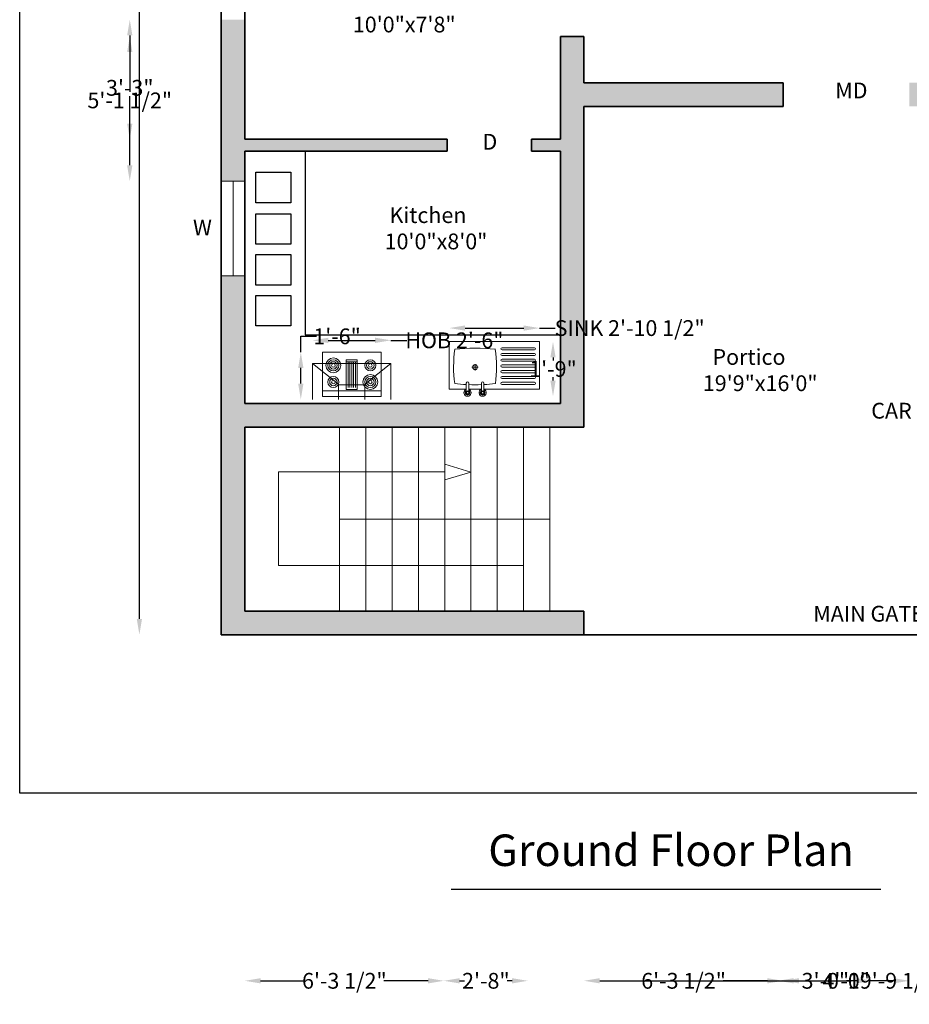
# Model space of a CAD drawing. Units: inches. Extents: x 1054 to 1577, y 4847 to 5610.
# Tile 1 of 5: x 1054 to 1393, y 4847 to 5221. Entities that reach past the tile are written whole.
import ezdxf

# ---------------------------------------------------------------- set-up
doc = ezdxf.new("R2010")
doc.units = ezdxf.units.IN
doc.header["$MEASUREMENT"] = 0
for name, color, linetype, lineweight in [('A-ANNO-DIMS', 2, 'Continuous', 18), ('A-ANNO-TEXT', 7, 'Continuous', 18), ('A-ANNO-TTLB', 7, 'Continuous', 25), ('A-AREA-IDEN', 7, 'Continuous', 18), ('A-EQPM', 8, 'Continuous', 18), ('A-FLOR-CASE', 7, 'Continuous', 25), ('A-FLOR-FIXT', 8, 'Continuous', 18), ('A-FLOR-STRS', 7, 'Continuous', 18), ('A-GLAZ', 4, 'Continuous', 18), ('A-WALL', 7, 'Continuous', 35)]:
    doc.layers.add(name, color=color, linetype=linetype, lineweight=lineweight)
doc.layers.add('A-WALL-PATT', color=240, linetype='Continuous', lineweight=13, true_color=0xed1f24)
doc.styles.get("Standard").update_dxf_attribs({"font": 'arial.ttf'})
doc.dimstyles.get("Standard").update_dxf_attribs({"dimtxt": 6, "dimasz": 6, "dimexe": 0.18, "dimexo": 0.0625, "dimgap": 0.09, "dimtad": 0, "dimtih": 1, "dimtoh": 1, "dimdec": 1, "dimzin": 0, "dimdsep": 46, "dimlunit": 3, "dimtxsty": 'Standard', "dimcen": 0.09, "dimse1": 1, "dimse2": 1, "dimadec": 0, "dimazin": 0, "dimtfac": 1, "dimtdec": 1, "dimtofl": 0, "dimtmove": 0, "dimatfit": 3, "dimfxl": 1, "dimtolj": 1, "dimtzin": 0, "dimarcsym": 0})

# ---------------------------------------------------------------- blocks, each defined once
blk = doc.blocks.new('chimmne')
for p, q in [((17.89, 6.07), (-18.11, 6.07)), ((-18.11, 6.07), (-18.11, -10.43)), ((-6.16, -3.43), (-18.11, 6.07)), ((5.94, -3.43), (17.89, 6.07)), ((17.89, 6.07), (17.89, -10.43)), ((-6.16, -3.43), (-6.16, -10.43)), ((5.94, -3.82), (-6.16, -3.82)), ((5.94, -3.43), (5.94, -10.43))]:
    blk.add_line(p, q)
for points in [[(-13.61, -9.12), (-13.61, 11.28), (13.39, 11.28), (13.39, -9.12)], [(-2.66, -5.87), (-2.66, 7.73), (2.44, 7.73), (2.44, -5.87)]]:
    blk.add_lwpolyline(points, close=True)
for points in [[(-2.66, 6.88), (2.44, 6.88)], [(-1.81, 6.88), (-1.81, -5.02)], [(-0.96, -5.02), (-0.96, 6.88)], [(-0.11, 6.88), (-0.11, -5.02)], [(0.74, -5.02), (0.74, 6.88)], [(1.59, 6.88), (1.59, -5.02)], [(13.39, -6.57), (-13.61, -6.57)]]:
    blk.add_lwpolyline(points)
for centre, radius in [((-8.55, 5.18), 3.4), ((-8.55, 5.18), 2.55), ((-8.55, 5.18), 1.7), ((-8.55, 5.18), 0.85), ((8.44, 5.18), 2.55), ((8.44, 5.18), 1.7), ((8.44, 5.18), 0.85), ((-8.55, -2.47), 2.55), ((8.44, -2.47), 3.4), ((8.44, -2.47), 2.55), ((-8.55, -2.47), 1.7), ((-8.55, -2.47), 0.85), ((8.44, -2.47), 1.7), ((8.44, -2.47), 0.85)]:
    blk.add_circle(centre, radius)
blk = doc.blocks.new('A$C799204C7')
for p, q in [((0, 34.2), (17.99, 34.2)), ((0, 0), (0, 34.2)), ((17.99, 13.08), (17.99, 34.2)), ((2.32, 20.01), (2.32, 32.27)), ((3.13, 20.01), (3.13, 32.27)), ((4.48, 20.01), (4.48, 32.27)), ((5.29, 20.01), (5.29, 32.27)), ((6.64, 20.01), (6.64, 32.27)), ((7.45, 20.01), (7.45, 32.27)), ((8.85, 20.01), (8.85, 32.27)), ((9.66, 20.01), (9.66, 32.27)), ((11.01, 20.01), (11.01, 32.27)), ((11.82, 20.01), (11.82, 32.27)), ((13.22, 20.01), (13.22, 32.27)), ((14.03, 20.01), (14.03, 32.27)), ((15.42, 20.01), (15.42, 32.27)), ((16.24, 20.01), (16.24, 32.27)), ((18.59, 13.08), (15.71, 13.08)), ((15.71, 12.17), (18.59, 12.17)), ((17.99, 7.36), (17.99, 12.17)), ((8.52, 9.77), (10.9, 9.77)), ((9.73, 11), (9.73, 8.54)), ((18.59, 7.36), (15.71, 7.36)), ((15.71, 6.45), (18.59, 6.45)), ((17.99, 0), (17.99, 6.45)), ((0, 0), (17.99, 0))]:
    blk.add_line(p, q)
for centre, radius in [((19.38, 12.62), 0.684), ((19.38, 12.62), 0.456), ((9.7, 9.77), 0.916), ((19.38, 6.91), 0.684), ((19.38, 6.91), 0.456)]:
    blk.add_circle(centre, radius)
for centre, radius, start, end in [((2.72, 32.27), 0.407, 0, 180), ((4.88, 32.27), 0.407, 0, 180), ((7.05, 32.27), 0.407, 0, 180), ((9.25, 32.27), 0.407, 0, 180), ((11.42, 32.27), 0.407, 0, 180), ((13.62, 32.27), 0.407, 0, 180), ((15.83, 32.27), 0.407, 0, 180), ((2.72, 20.01), 0.407, 180, 0), ((4.88, 20.01), 0.407, 180, 0), ((7.05, 20.01), 0.407, 180, 0), ((9.25, 20.01), 0.407, 180, 0), ((11.42, 20.01), 0.407, 180, 0), ((13.62, 20.01), 0.407, 180, 0), ((15.83, 20.01), 0.407, 180, 0), ((67.33, 9.77), 64.88, 173.1952, 186.8048), ((9.53, -30.19), 48.1, 82.3437, 97.8966), ((-48.51, 9.77), 64.88, 2.9208, 6.8048), ((15.71, 12.62), 0.456, 90, 270), ((-48.51, 9.77), 64.88, 357.8723, 2.115), ((19.38, 12.62), 1.37, 199.6514, 160.3603), ((19.38, 12.62), 0.911, 210.3431, 149.7554), ((19.38, 6.91), 1.37, 199.6514, 160.3603), ((19.38, 6.91), 0.911, 210.3431, 149.7554), ((15.71, 6.91), 0.456, 90, 270), ((-48.51, 9.77), 64.88, 353.1952, 357.0665), ((9.53, 49.73), 48.1, 262.1034, 277.6563)]:
    blk.add_arc(centre, radius, start, end)
blk = doc.blocks.new('*D5')
at = {"layer": 'A-ANNO-DIMS', "color": 0, "lineweight": -2, "transparency": 16777216}
for p, q in [((1099.63, 5521.48), (1099.63, 5260.62)), ((1099.63, 4993.48), (1099.63, 5254.34))]:
    blk.add_line(p, q, dxfattribs=at)
at = {"layer": 'A-ANNO-DIMS', "color": 0, "transparency": 16777216}
for points in [[(1098.63, 5521.48), (1100.63, 5521.48), (1099.63, 5527.48)], [(1098.63, 4993.48), (1100.63, 4993.48), (1099.63, 4987.48)]]:
    blk.add_solid(points, dxfattribs=at)
at = {"layer": 'Defpoints', "color": 0, "transparency": 16777216}
for p in [(1130.77, 5527.48), (1099.63, 4987.48), (1130.77, 4987.48)]:
    blk.add_point(p, dxfattribs=at)
at = {"layer": 'A-ANNO-DIMS', "color": 0, "transparency": 16777216, "insert": (1099.63, 5257.48), "char_height": 6, "attachment_point": 5}
blk.add_mtext("\\A1;45'", dxfattribs=at)
blk = doc.blocks.new('WINDOW-36IN')
for p, q in [((0, 9), (0, 0)), ((36, 9), (0, 9)), ((36, 0), (36, 9)), ((36, 4.5), (0, 4.5)), ((0, 0), (36, 0))]:
    blk.add_line(p, q)
blk = doc.blocks.new('*D18')
at = {"layer": 'A-ANNO-DIMS', "color": 0, "lineweight": -2, "transparency": 16777216}
for p, q in [((1171.51, 5099.49), (1189.32, 5099.49)), ((1195.32, 5099.49), (1201.32, 5099.49))]:
    blk.add_line(p, q, dxfattribs=at)
at = {"layer": 'A-ANNO-DIMS', "color": 0, "transparency": 16777216}
for points in [[(1171.51, 5100.49), (1171.51, 5098.49), (1165.51, 5099.49)], [(1189.32, 5100.49), (1189.32, 5098.49), (1195.32, 5099.49)]]:
    blk.add_solid(points, dxfattribs=at)
at = {"layer": 'Defpoints', "color": 0, "transparency": 16777216}
for p in [(1195.32, 5099.49), (1165.51, 5095.02), (1195.32, 5095.02)]:
    blk.add_point(p, dxfattribs=at)
at = {"layer": 'A-ANNO-DIMS', "color": 0, "transparency": 16777216, "insert": (1219.47, 5099.49), "char_height": 6, "attachment_point": 5}
blk.add_mtext('\\A1;HOB 2\'-6"', dxfattribs=at)
blk = doc.blocks.new('*D19')
at = {"layer": 'A-ANNO-DIMS', "color": 0, "lineweight": -2, "transparency": 16777216}
for p, q in [((1161.04, 5095.02), (1161.04, 5101.02)), ((1161.04, 5101.02), (1167.04, 5101.02)), ((1161.04, 5083.04), (1161.04, 5089.02))]:
    blk.add_line(p, q, dxfattribs=at)
at = {"layer": 'A-ANNO-DIMS', "color": 0, "transparency": 16777216}
for points in [[(1160.04, 5089.02), (1162.04, 5089.02), (1161.04, 5095.02)], [(1160.04, 5083.04), (1162.04, 5083.04), (1161.04, 5077.04)]]:
    blk.add_solid(points, dxfattribs=at)
at = {"layer": 'Defpoints', "color": 0, "transparency": 16777216}
for p in [(1161.04, 5095.02), (1165.51, 5095.02), (1165.51, 5077.04)]:
    blk.add_point(p, dxfattribs=at)
at = {"layer": 'A-ANNO-DIMS', "color": 0, "transparency": 16777216, "insert": (1174.83, 5101.02), "char_height": 6, "attachment_point": 5}
blk.add_mtext('\\A1;1\'-6"', dxfattribs=at)
blk = doc.blocks.new('*D20')
at = {"layer": 'A-ANNO-DIMS', "color": 0, "lineweight": -2, "transparency": 16777216}
for p, q in [((1223.53, 5104.16), (1245.84, 5104.16)), ((1251.84, 5104.16), (1257.84, 5104.16))]:
    blk.add_line(p, q, dxfattribs=at)
at = {"layer": 'A-ANNO-DIMS', "color": 0, "transparency": 16777216}
for points in [[(1223.53, 5105.16), (1223.53, 5103.16), (1217.53, 5104.16)], [(1245.84, 5105.16), (1245.84, 5103.16), (1251.84, 5104.16)]]:
    blk.add_solid(points, dxfattribs=at)
at = {"layer": 'Defpoints', "color": 0, "transparency": 16777216}
for p in [(1251.84, 5104.16), (1217.53, 5099.01), (1251.84, 5099.01)]:
    blk.add_point(p, dxfattribs=at)
at = {"layer": 'A-ANNO-DIMS', "color": 0, "transparency": 16777216, "insert": (1286.15, 5104.16), "char_height": 6, "attachment_point": 5}
blk.add_mtext('\\A1;SINK 2\'-10 1/2"', dxfattribs=at)
blk = doc.blocks.new('*D21')
at = {"layer": 'A-ANNO-DIMS', "color": 0, "lineweight": -2, "transparency": 16777216}
for p, q in [((1256.98, 5093.01), (1256.98, 5091.76)), ((1256.98, 5084.2), (1256.98, 5085.45))]:
    blk.add_line(p, q, dxfattribs=at)
at = {"layer": 'A-ANNO-DIMS', "color": 0, "transparency": 16777216}
for points in [[(1255.98, 5093.01), (1257.98, 5093.01), (1256.98, 5099.01)], [(1255.98, 5084.2), (1257.98, 5084.2), (1256.98, 5078.2)]]:
    blk.add_solid(points, dxfattribs=at)
at = {"layer": 'Defpoints', "color": 0, "transparency": 16777216}
for p in [(1251.84, 5099.01), (1251.84, 5078.2), (1256.98, 5078.2)]:
    blk.add_point(p, dxfattribs=at)
at = {"layer": 'A-ANNO-DIMS', "color": 0, "transparency": 16777216, "insert": (1256.98, 5088.6), "char_height": 6, "attachment_point": 5}
blk.add_mtext('\\A1;1\'-9"', dxfattribs=at)
blk = doc.blocks.new('*D22')
at = {"layer": 'A-ANNO-DIMS', "color": 0, "lineweight": -2, "transparency": 16777216}
for p, q in [((1397.97, 5125.61), (1397.97, 5075.91)), ((1397.97, 5019.83), (1397.97, 5069.53))]:
    blk.add_line(p, q, dxfattribs=at)
at = {"layer": 'A-ANNO-DIMS', "color": 0, "transparency": 16777216}
for points in [[(1396.97, 5125.61), (1398.97, 5125.61), (1397.97, 5131.61)], [(1396.97, 5019.83), (1398.97, 5019.83), (1397.97, 5013.83)]]:
    blk.add_solid(points, dxfattribs=at)
at = {"layer": 'Defpoints', "color": 0, "transparency": 16777216}
for p in [(1415.63, 5131.61), (1397.97, 5013.83), (1415.63, 5013.83)]:
    blk.add_point(p, dxfattribs=at)
at = {"layer": 'A-ANNO-DIMS', "color": 0, "transparency": 16777216, "insert": (1397.97, 5072.72), "char_height": 6, "attachment_point": 5}
blk.add_mtext('\\A1;CAR 9\'-10"', dxfattribs=at)
blk = doc.blocks.new('*D24')
at = {"layer": 'A-ANNO-DIMS', "color": 0, "lineweight": -2, "transparency": 16777216}
for p, q in [((1350.52, 4855.83), (1360.34, 4855.83)), ((1386.52, 4855.83), (1376.71, 4855.83))]:
    blk.add_line(p, q, dxfattribs=at)
at = {"layer": 'A-ANNO-DIMS', "color": 0, "transparency": 16777216}
for points in [[(1350.52, 4856.83), (1350.52, 4854.83), (1344.52, 4855.83)], [(1386.52, 4856.83), (1386.52, 4854.83), (1392.52, 4855.83)]]:
    blk.add_solid(points, dxfattribs=at)
at = {"layer": 'Defpoints', "color": 0, "transparency": 16777216}
for p in [(1344.52, 5188.48), (1392.52, 5188.48), (1392.52, 4855.83)]:
    blk.add_point(p, dxfattribs=at)
at = {"layer": 'A-ANNO-DIMS', "color": 0, "transparency": 16777216, "insert": (1368.52, 4855.83), "char_height": 6, "attachment_point": 5}
blk.add_mtext('\\A1;4\'-0"', dxfattribs=at)
blk = doc.blocks.new('*D25')
at = {"layer": 'A-ANNO-DIMS', "color": 0, "lineweight": -2, "transparency": 16777216}
for p, q in [((1348.59, 4855.83), (1352.52, 4855.83)), ((1372.59, 4855.83), (1368.65, 4855.83))]:
    blk.add_line(p, q, dxfattribs=at)
at = {"layer": 'A-ANNO-DIMS', "color": 0, "transparency": 16777216}
for points in [[(1348.59, 4856.83), (1348.59, 4854.83), (1342.59, 4855.83)], [(1372.59, 4856.83), (1372.59, 4854.83), (1378.59, 4855.83)]]:
    blk.add_solid(points, dxfattribs=at)
at = {"layer": 'Defpoints', "color": 0, "transparency": 16777216}
for p in [(1342.59, 5389.48), (1378.59, 5389.48), (1378.59, 4855.83)]:
    blk.add_point(p, dxfattribs=at)
at = {"layer": 'A-ANNO-DIMS', "color": 0, "transparency": 16777216, "insert": (1360.59, 4855.83), "char_height": 6, "attachment_point": 5}
blk.add_mtext('\\A1;3\'-0"', dxfattribs=at)
blk = doc.blocks.new('*D26')
at = {"layer": 'A-ANNO-DIMS', "color": 0, "lineweight": -2, "transparency": 16777216}
for p, q in [((1221.44, 4855.83), (1223.32, 4855.83)), ((1241.44, 4855.83), (1239.56, 4855.83))]:
    blk.add_line(p, q, dxfattribs=at)
at = {"layer": 'A-ANNO-DIMS', "color": 0, "transparency": 16777216}
for points in [[(1221.44, 4856.83), (1221.44, 4854.83), (1215.44, 4855.83)], [(1241.44, 4856.83), (1241.44, 4854.83), (1247.44, 4855.83)]]:
    blk.add_solid(points, dxfattribs=at)
at = {"layer": 'Defpoints', "color": 0, "transparency": 16777216}
for p in [(1215.44, 5324.98), (1247.44, 5324.98), (1247.44, 4855.83)]:
    blk.add_point(p, dxfattribs=at)
at = {"layer": 'A-ANNO-DIMS', "color": 0, "transparency": 16777216, "insert": (1231.44, 4855.83), "char_height": 6, "attachment_point": 5}
blk.add_mtext('\\A1;2\'-8"', dxfattribs=at)
blk = doc.blocks.new('*D27')
at = {"layer": 'A-ANNO-DIMS', "color": 0, "lineweight": -2, "transparency": 16777216}
for p, q in [((1550.07, 5060.48), (1550.07, 5034.64)), ((1550.07, 5002.48), (1550.07, 5028.33))]:
    blk.add_line(p, q, dxfattribs=at)
at = {"layer": 'A-ANNO-DIMS', "color": 0, "transparency": 16777216}
for points in [[(1549.07, 5060.48), (1551.07, 5060.48), (1550.07, 5066.48)], [(1549.07, 5002.48), (1551.07, 5002.48), (1550.07, 4996.48)]]:
    blk.add_solid(points, dxfattribs=at)
at = {"layer": 'Defpoints', "color": 0, "transparency": 16777216}
for p in [(1139.77, 5066.48), (1550.07, 5066.48), (1139.77, 4996.48)]:
    blk.add_point(p, dxfattribs=at)
at = {"layer": 'A-ANNO-DIMS', "color": 0, "transparency": 16777216, "insert": (1550.07, 5031.48), "char_height": 6, "attachment_point": 5}
blk.add_mtext('\\A1;5\'-10"', dxfattribs=at)
blk = doc.blocks.new('*D28')
at = {"layer": 'A-ANNO-DIMS', "color": 0, "lineweight": -2, "transparency": 16777216}
for p, q in [((1274.77, 4855.83), (1370.42, 4855.83)), ((1500.27, 4855.83), (1404.63, 4855.83))]:
    blk.add_line(p, q, dxfattribs=at)
at = {"layer": 'A-ANNO-DIMS', "color": 0, "transparency": 16777216}
for points in [[(1274.77, 4856.83), (1274.77, 4854.83), (1268.77, 4855.83)], [(1500.27, 4856.83), (1500.27, 4854.83), (1506.27, 4855.83)]]:
    blk.add_solid(points, dxfattribs=at)
at = {"layer": 'Defpoints', "color": 0, "transparency": 16777216}
for p in [(1268.77, 4987.48), (1506.27, 4987.48), (1506.27, 4855.83)]:
    blk.add_point(p, dxfattribs=at)
at = {"layer": 'A-ANNO-DIMS', "color": 0, "transparency": 16777216, "insert": (1387.52, 4855.83), "char_height": 6, "attachment_point": 5}
blk.add_mtext('\\A1;19\'-9 1/2"', dxfattribs=at)
blk = doc.blocks.new('*D32')
at = {"layer": 'A-ANNO-DIMS', "color": 0, "lineweight": -2, "transparency": 16777216}
for p, q in [((1095.97, 5215.48), (1095.97, 5193.98)), ((1095.97, 5166.09), (1095.97, 5187.59))]:
    blk.add_line(p, q, dxfattribs=at)
at = {"layer": 'A-ANNO-DIMS', "color": 0, "transparency": 16777216}
for points in [[(1094.97, 5215.48), (1096.97, 5215.48), (1095.97, 5221.48)], [(1094.97, 5166.09), (1096.97, 5166.09), (1095.97, 5160.09)]]:
    blk.add_solid(points, dxfattribs=at)
at = {"layer": 'Defpoints', "color": 0, "transparency": 16777216}
for p in [(1095.97, 5221.48), (1130.77, 5221.48), (1130.77, 5160.09)]:
    blk.add_point(p, dxfattribs=at)
at = {"layer": 'A-ANNO-DIMS', "color": 0, "transparency": 16777216, "insert": (1095.97, 5190.78), "char_height": 6, "attachment_point": 5}
blk.add_mtext('\\A1;5\'-1 1/2"', dxfattribs=at)
blk = doc.blocks.new('*D38')
at = {"layer": 'A-ANNO-DIMS', "color": 0, "lineweight": -2, "transparency": 16777216}
for p, q in [((1274.77, 4855.83), (1291.58, 4855.83)), ((1338.52, 4855.83), (1321.72, 4855.83))]:
    blk.add_line(p, q, dxfattribs=at)
at = {"layer": 'A-ANNO-DIMS', "color": 0, "transparency": 16777216}
for points in [[(1274.77, 4856.83), (1274.77, 4854.83), (1268.77, 4855.83)], [(1338.52, 4856.83), (1338.52, 4854.83), (1344.52, 4855.83)]]:
    blk.add_solid(points, dxfattribs=at)
at = {"layer": 'Defpoints', "color": 0, "transparency": 16777216}
for p in [(1268.77, 5188.48), (1344.52, 5188.48), (1344.52, 4855.83)]:
    blk.add_point(p, dxfattribs=at)
at = {"layer": 'A-ANNO-DIMS', "color": 0, "transparency": 16777216, "insert": (1306.65, 4855.83), "char_height": 6, "attachment_point": 5}
blk.add_mtext('\\A1;6\'-3 1/2"', dxfattribs=at)
blk = doc.blocks.new('*D39')
at = {"layer": 'A-ANNO-DIMS', "color": 0, "lineweight": -2, "transparency": 16777216}
for p, q in [((1181.77, 5562.28), (1207.69, 5562.28)), ((1249.77, 5562.28), (1223.86, 5562.28))]:
    blk.add_line(p, q, dxfattribs=at)
at = {"layer": 'A-ANNO-DIMS', "color": 0, "transparency": 16777216}
for points in [[(1181.77, 5563.28), (1181.77, 5561.28), (1175.77, 5562.28)], [(1249.77, 5563.28), (1249.77, 5561.28), (1255.77, 5562.28)]]:
    blk.add_solid(points, dxfattribs=at)
at = {"layer": 'Defpoints', "color": 0, "transparency": 16777216}
for p in [(1255.77, 5562.28), (1175.77, 4996.48), (1255.77, 4996.48)]:
    blk.add_point(p, dxfattribs=at)
at = {"layer": 'A-ANNO-DIMS', "color": 0, "transparency": 16777216, "insert": (1215.77, 5562.28), "char_height": 6, "attachment_point": 5}
blk.add_mtext('\\A1;6\'-8"', dxfattribs=at)
blk = doc.blocks.new('*D40')
at = {"layer": 'A-ANNO-DIMS', "color": 0, "lineweight": -2, "transparency": 16777216}
for p, q in [((1145.77, 5562.28), (1149.71, 5562.28)), ((1169.77, 5562.28), (1165.84, 5562.28))]:
    blk.add_line(p, q, dxfattribs=at)
at = {"layer": 'A-ANNO-DIMS', "color": 0, "transparency": 16777216}
for points in [[(1145.77, 5563.28), (1145.77, 5561.28), (1139.77, 5562.28)], [(1169.77, 5563.28), (1169.77, 5561.28), (1175.77, 5562.28)]]:
    blk.add_solid(points, dxfattribs=at)
at = {"layer": 'Defpoints', "color": 0, "transparency": 16777216}
for p in [(1175.77, 5562.28), (1139.77, 4996.48), (1175.77, 4996.48)]:
    blk.add_point(p, dxfattribs=at)
at = {"layer": 'A-ANNO-DIMS', "color": 0, "transparency": 16777216, "insert": (1157.77, 5562.28), "char_height": 6, "attachment_point": 5}
blk.add_mtext('\\A1;3\'-0"', dxfattribs=at)
blk = doc.blocks.new('*D41')
at = {"layer": 'A-ANNO-DIMS', "color": 0, "lineweight": -2, "transparency": 16777216}
for p, q in [((1239.77, 5562.28), (1233.77, 5562.28)), ((1261.77, 5562.28), (1267.77, 5562.28))]:
    blk.add_line(p, q, dxfattribs=at)
at = {"layer": 'A-ANNO-DIMS', "color": 0, "transparency": 16777216}
for points in [[(1239.77, 5563.28), (1239.77, 5561.28), (1245.77, 5562.28)], [(1261.77, 5563.28), (1261.77, 5561.28), (1255.77, 5562.28)]]:
    blk.add_solid(points, dxfattribs=at)
at = {"layer": 'Defpoints', "color": 0, "transparency": 16777216}
for p in [(1255.77, 5562.28), (1245.77, 4996.48), (1255.77, 4996.48)]:
    blk.add_point(p, dxfattribs=at)
at = {"layer": 'A-ANNO-DIMS', "color": 0, "transparency": 16777216, "insert": (1278.17, 5562.28), "char_height": 6, "attachment_point": 5}
blk.add_mtext('\\A1;0\'-10"', dxfattribs=at)
blk = doc.blocks.new('*D42')
at = {"layer": 'A-ANNO-DIMS', "color": 0, "lineweight": -2, "transparency": 16777216}
for p, q in [((1095.97, 5209.14), (1095.97, 5198.72)), ((1095.97, 5181.98), (1095.97, 5192.41))]:
    blk.add_line(p, q, dxfattribs=at)
at = {"layer": 'A-ANNO-DIMS', "color": 0, "transparency": 16777216}
for points in [[(1094.97, 5209.14), (1096.97, 5209.14), (1095.97, 5215.14)], [(1094.97, 5181.98), (1096.97, 5181.98), (1095.97, 5175.98)]]:
    blk.add_solid(points, dxfattribs=at)
at = {"layer": 'Defpoints', "color": 0, "transparency": 16777216}
for p in [(1095.97, 5215.14), (1259.77, 5215.14), (1259.77, 5175.98)]:
    blk.add_point(p, dxfattribs=at)
at = {"layer": 'A-ANNO-DIMS', "color": 0, "transparency": 16777216, "insert": (1095.97, 5195.56), "char_height": 6, "attachment_point": 5}
blk.add_mtext('\\A1;3\'-3"', dxfattribs=at)
blk = doc.blocks.new('*D46')
at = {"layer": 'A-ANNO-DIMS', "color": 0, "lineweight": -2, "transparency": 16777216}
for p, q in [((1145.77, 4855.83), (1162.54, 4855.83)), ((1209.44, 4855.83), (1192.68, 4855.83))]:
    blk.add_line(p, q, dxfattribs=at)
at = {"layer": 'A-ANNO-DIMS', "color": 0, "transparency": 16777216}
for points in [[(1145.77, 4856.83), (1145.77, 4854.83), (1139.77, 4855.83)], [(1209.44, 4856.83), (1209.44, 4854.83), (1215.44, 4855.83)]]:
    blk.add_solid(points, dxfattribs=at)
at = {"layer": 'Defpoints', "color": 0, "transparency": 16777216}
for p in [(1139.77, 5324.98), (1215.44, 5324.98), (1215.44, 4855.83)]:
    blk.add_point(p, dxfattribs=at)
at = {"layer": 'A-ANNO-DIMS', "color": 0, "transparency": 16777216, "insert": (1177.61, 4855.83), "char_height": 6, "attachment_point": 5}
blk.add_mtext('\\A1;6\'-3 1/2"', dxfattribs=at)
blk = doc.blocks.new('*D47')
at = {"layer": 'A-ANNO-DIMS', "color": 0, "lineweight": -2, "transparency": 16777216}
for p, q in [((1242.78, 5562.28), (1236.78, 5562.28)), ((1265.77, 5562.28), (1271.77, 5562.28))]:
    blk.add_line(p, q, dxfattribs=at)
at = {"layer": 'A-ANNO-DIMS', "color": 0, "transparency": 16777216}
for points in [[(1242.78, 5563.28), (1242.78, 5561.28), (1248.78, 5562.28)], [(1265.77, 5563.28), (1265.77, 5561.28), (1259.77, 5562.28)]]:
    blk.add_solid(points, dxfattribs=at)
at = {"layer": 'Defpoints', "color": 0, "transparency": 16777216}
for p in [(1259.77, 5562.28), (1248.78, 5175.98), (1259.77, 5175.98)]:
    blk.add_point(p, dxfattribs=at)
at = {"layer": 'A-ANNO-DIMS', "color": 0, "transparency": 16777216, "insert": (1282.17, 5562.28), "char_height": 6, "attachment_point": 5}
blk.add_mtext('\\A1;0\'-11"', dxfattribs=at)
blk = doc.blocks.new('*D53')
at = {"layer": 'A-ANNO-DIMS', "color": 0, "lineweight": -2, "transparency": 16777216}
for p, q in [((1145.77, 5562.28), (1159.51, 5562.28)), ((1165.51, 5562.28), (1171.51, 5562.28))]:
    blk.add_line(p, q, dxfattribs=at)
at = {"layer": 'A-ANNO-DIMS', "color": 0, "transparency": 16777216}
for points in [[(1145.77, 5563.28), (1145.77, 5561.28), (1139.77, 5562.28)], [(1159.51, 5563.28), (1159.51, 5561.28), (1165.51, 5562.28)]]:
    blk.add_solid(points, dxfattribs=at)
at = {"layer": 'Defpoints', "color": 0, "transparency": 16777216}
for p in [(1165.51, 5562.28), (1165.51, 5077.04), (1139.77, 5075.48)]:
    blk.add_point(p, dxfattribs=at)
at = {"layer": 'A-ANNO-DIMS', "color": 0, "transparency": 16777216, "insert": (1186.62, 5562.28), "char_height": 6, "attachment_point": 5}
blk.add_mtext('\\A1;2\'-1 1/2"', dxfattribs=at)
blk = doc.blocks.new('*D54')
at = {"layer": 'A-ANNO-DIMS', "color": 0, "lineweight": -2, "transparency": 16777216}
for p, q in [((1245.84, 5562.28), (1239.84, 5562.28)), ((1265.77, 5562.28), (1271.77, 5562.28))]:
    blk.add_line(p, q, dxfattribs=at)
at = {"layer": 'A-ANNO-DIMS', "color": 0, "transparency": 16777216}
for points in [[(1245.84, 5563.28), (1245.84, 5561.28), (1251.84, 5562.28)], [(1265.77, 5563.28), (1265.77, 5561.28), (1259.77, 5562.28)]]:
    blk.add_solid(points, dxfattribs=at)
at = {"layer": 'Defpoints', "color": 0, "transparency": 16777216}
for p in [(1259.77, 5562.28), (1251.84, 5080.96), (1259.77, 5075.48)]:
    blk.add_point(p, dxfattribs=at)
at = {"layer": 'A-ANNO-DIMS', "color": 0, "transparency": 16777216, "insert": (1279.84, 5562.28), "char_height": 6, "attachment_point": 5}
blk.add_mtext('\\A1;0\'-8"', dxfattribs=at)
blk = doc.blocks.new('*D55')
at = {"layer": 'A-ANNO-DIMS', "color": 0, "lineweight": -2, "transparency": 16777216}
for p, q in [((1550.07, 5095.58), (1550.07, 5091.63)), ((1550.07, 5081.48), (1550.07, 5085.43))]:
    blk.add_line(p, q, dxfattribs=at)
at = {"layer": 'A-ANNO-DIMS', "color": 0, "transparency": 16777216}
for points in [[(1549.07, 5095.58), (1551.07, 5095.58), (1550.07, 5101.58)], [(1549.07, 5081.48), (1551.07, 5081.48), (1550.07, 5075.48)]]:
    blk.add_solid(points, dxfattribs=at)
at = {"layer": 'Defpoints', "color": 0, "transparency": 16777216}
for p in [(1259.77, 5101.58), (1550.07, 5101.58), (1259.77, 5075.48)]:
    blk.add_point(p, dxfattribs=at)
at = {"layer": 'A-ANNO-DIMS', "color": 0, "transparency": 16777216, "insert": (1550.07, 5088.53), "char_height": 6, "attachment_point": 5}
blk.add_mtext('\\A1;2\'-2"', dxfattribs=at)

msp = doc.modelspace()

# ---------------------------------------------------------------- hatches: boundary and pattern name
at = {"layer": 'A-WALL-PATT'}
h = msp.add_hatch(color=256, dxfattribs=at)
h.dxf.hatch_style = 1
h.paths.add_polyline_path([(1213.08, 5527.48), (1130.77, 5527.48), (1130.77, 5375.41), (1139.77, 5375.41), (1139.77, 5518.48), (1213.08, 5518.48)])
h.paths.add_polyline_path([(1470.27, 5527.48), (1383.75, 5527.48), (1383.75, 5518.48), (1457.77, 5518.48), (1457.77, 5446.33), (1462.27, 5446.33), (1462.27, 5518.48), (1470.27, 5518.48)], flags=17)
h.paths.add_polyline_path([(1515.27, 5527.48), (1506.27, 5527.48), (1506.27, 5518.48), (1506.27, 5398.48), (1462.27, 5398.48), (1462.27, 5414.33), (1457.77, 5414.33), (1457.77, 5398.48), (1378.59, 5398.48), (1378.59, 5389.48), (1506.27, 5389.48), (1506.27, 5365.03), (1515.27, 5365.03)])
h.paths.add_polyline_path([(1515.27, 5329.03), (1506.27, 5329.03), (1506.27, 5255.01), (1515.27, 5255.01)])
h.paths.add_polyline_path([(1515.27, 5219.01), (1506.27, 5219.01), (1506.27, 5197.48), (1392.52, 5197.48), (1392.52, 5188.48), (1515.27, 5188.48)])
h.paths.add_polyline_path([(1344.52, 5197.48), (1268.77, 5197.48), (1268.77, 5215.14), (1259.77, 5215.14), (1259.77, 5175.98), (1248.78, 5175.98), (1248.78, 5171.48), (1259.77, 5171.48), (1259.77, 5075.48), (1139.77, 5075.48), (1139.77, 5124.09), (1130.77, 5124.09), (1130.77, 4987.48), (1268.77, 4987.48), (1268.77, 4996.48), (1139.77, 4996.48), (1139.77, 5066.48), (1175.77, 5066.48), (1268.77, 5066.48), (1268.77, 5188.48), (1344.52, 5188.48)])
h.paths.add_polyline_path([(1216.78, 5175.98), (1139.77, 5175.98), (1139.77, 5221.48), (1130.77, 5221.48), (1130.77, 5160.09), (1139.77, 5160.09), (1139.77, 5171.48), (1216.78, 5171.48)])
h.paths.add_polyline_path([(1268.77, 5339.26), (1259.77, 5339.26), (1259.77, 5329.48), (1247.44, 5329.48), (1247.44, 5324.98), (1259.77, 5324.98), (1259.77, 5276.98), (1139.77, 5276.98), (1139.77, 5281.9), (1130.77, 5281.9), (1130.77, 5257.48), (1139.77, 5257.48), (1139.77, 5267.98), (1259.77, 5267.98), (1259.77, 5251.14), (1268.77, 5251.14)])
h.paths.add_polyline_path([(1139.77, 5339.41), (1130.77, 5339.41), (1130.77, 5317.9), (1139.77, 5317.9), (1139.77, 5324.98), (1215.44, 5324.98), (1215.44, 5329.48), (1139.77, 5329.48)])
h.paths.add_polyline_path([(1280.67, 5389.48), (1280.67, 5391.1), (1320.18, 5391.1), (1320.18, 5389.48), (1342.59, 5389.48), (1342.59, 5398.48), (1268.77, 5398.48), (1268.77, 5518.48), (1347.75, 5518.48), (1347.75, 5527.48), (1249.08, 5527.48), (1249.08, 5518.48), (1259.77, 5518.48), (1259.77, 5375.26), (1268.77, 5375.26), (1268.77, 5389.48)])

# ---------------------------------------------------------------- linework, layer by layer
at = {"layer": 'A-ANNO-TTLB'}
msp.add_line((1218.19, 4890.63), (1381.75, 4890.63), dxfattribs=at)
msp.add_lwpolyline([(1054.1, 5610.1), (1577.31, 5610.1), (1577.31, 4927.21), (1054.1, 4927.21)], close=True, dxfattribs=at)
at = {"layer": 'A-FLOR-CASE'}
for p, q in [((1162.64, 5171.48), (1162.64, 5101.58)), ((1162.64, 5101.58), (1259.77, 5101.58))]:
    msp.add_line(p, q, dxfattribs=at)
for points in [[(1143.87, 5163.43), (1157.21, 5163.43), (1157.21, 5151.83), (1143.87, 5151.83)], [(1143.87, 5147.63), (1157.21, 5147.63), (1157.21, 5136.03), (1143.87, 5136.03)], [(1143.87, 5132.14), (1157.21, 5132.14), (1157.21, 5120.53), (1143.87, 5120.53)], [(1143.87, 5116.58), (1157.21, 5116.58), (1157.21, 5104.98), (1143.87, 5104.98)]]:
    msp.add_lwpolyline(points, close=True, dxfattribs=at)
at = {"layer": 'A-FLOR-STRS'}
for p, q in [((1139.77, 5066.48), (1175.77, 5066.48)), ((1175.77, 5066.48), (1175.77, 4996.48)), ((1185.77, 5066.48), (1185.77, 4996.48)), ((1195.77, 5066.48), (1195.77, 4996.48)), ((1205.77, 5066.48), (1205.77, 4996.48)), ((1215.77, 5066.48), (1215.77, 4996.48)), ((1225.77, 5066.48), (1225.77, 4996.48)), ((1235.77, 5066.48), (1235.77, 4996.48)), ((1245.77, 5066.48), (1245.77, 4996.48)), ((1255.77, 5066.48), (1255.77, 4996.48)), ((1215.77, 5052.42), (1225.77, 5049.39)), ((1215.77, 5052.42), (1215.77, 5046.42)), ((1152.56, 5013.77), (1152.56, 5049.42)), ((1152.56, 5049.42), (1215.77, 5049.42)), ((1215.77, 5046.42), (1225.77, 5049.39)), ((1255.77, 5031.48), (1175.77, 5031.48)), ((1245.77, 5013.77), (1152.56, 5013.77))]:
    msp.add_line(p, q, dxfattribs=at)
at = {"layer": 'A-WALL'}
for p, q in [((1130.77, 5527.48), (1130.77, 4987.48)), ((1139.77, 5267.98), (1139.77, 5175.98)), ((1268.77, 5215.14), (1259.77, 5215.14)), ((1259.77, 5215.14), (1259.77, 5175.98)), ((1268.77, 5215.14), (1268.77, 5197.48)), ((1268.77, 5197.48), (1344.52, 5197.48)), ((1344.52, 5197.48), (1344.52, 5188.48)), ((1268.77, 5188.48), (1344.52, 5188.48)), ((1268.77, 5188.48), (1268.77, 5066.48)), ((1139.77, 5175.98), (1216.78, 5175.98)), ((1216.78, 5171.48), (1216.78, 5175.98)), ((1248.78, 5175.98), (1248.78, 5171.48)), ((1248.78, 5175.98), (1259.77, 5175.98)), ((1139.77, 5171.48), (1216.78, 5171.48)), ((1139.77, 5171.48), (1139.77, 5075.48)), ((1248.78, 5171.48), (1259.77, 5171.48)), ((1259.77, 5171.48), (1259.77, 5075.48)), ((1139.77, 5075.48), (1259.77, 5075.48)), ((1139.77, 5066.48), (1268.77, 5066.48)), ((1139.77, 5066.48), (1139.77, 4996.48)), ((1139.77, 4996.48), (1268.77, 4996.48)), ((1268.77, 4996.48), (1268.77, 4987.48)), ((1130.77, 4987.48), (1515.27, 4987.48))]:
    msp.add_line(p, q, dxfattribs=at)

# ---------------------------------------------------------------- block references
at = {"layer": 'A-EQPM', "xscale": 0.8280321260258986, "yscale": 0.8280321260258986, "zscale": 0.8280321260258986}
msp.add_blockref('chimmne', (1180.51, 5085.68), dxfattribs=at)
at = {"layer": 'A-FLOR-FIXT', "xscale": 1.0032, "yscale": 1.0032, "zscale": 1.0032, "rotation": 270}
msp.add_blockref('A$C799204C7', (1217.53, 5099.01), dxfattribs=at)
at = {"layer": 'A-GLAZ', "rotation": 269.9999999999954}
msp.add_blockref('WINDOW-36IN', (1130.77, 5160.09), dxfattribs=at)

# ---------------------------------------------------------------- texts
at = {"layer": 'A-ANNO-TEXT', "char_height": 6, "attachment_point": 1}
for s, width, insert in [('MD', 9.6402, (1364.34, 5197.57)), ('D', 9.0631, (1230.14, 5178.04)), ('W', 11.4277, (1120.02, 5145.4)), ('MAIN GATE', 65.9178, (1355.99, 4998.48))]:
    msp.add_mtext_dynamic_manual_height_columns(s, width=width, gutter_width=30, heights=[0], dxfattribs=dict(at, insert=insert))
at = {"layer": 'A-ANNO-TTLB', "insert": (1232.35, 4911.5), "char_height": 12, "attachment_point": 1}
msp.add_mtext_dynamic_manual_height_columns('Ground Floor Plan', width=222.348, gutter_width=30, heights=[0], dxfattribs=at)
at = {"layer": 'A-AREA-IDEN', "char_height": 6, "attachment_point": 1}
for s, width, insert in [('  Dining\\P10\'0"x7\'8"', 62.8209, (1180.83, 5232.65)), (' Kitchen\\P10\'0"x8\'0"', 57.2112, (1192.92, 5150.13)), ('  Portico\\P19\'9"x16\'0"', 68.2028, (1313.97, 5096.17))]:
    msp.add_mtext_dynamic_manual_height_columns(s, width=width, gutter_width=30, heights=[0], dxfattribs=dict(at, insert=insert))

# ---------------------------------------------------------------- dimensions: what is measured, and where the dimension line sits
at = {"layer": 'A-ANNO-DIMS'}
for base, p1, p2, picture, middle in [((1165.51, 5562.28), (1139.77, 5075.48), (1165.51, 5077.04), '*D53', (1186.62, 5562.28)), ((1175.77, 5562.28), (1139.77, 4996.48), (1175.77, 4996.48), '*D40', (1157.77, 5562.28)), ((1255.77, 5562.28), (1175.77, 4996.48), (1255.77, 4996.48), '*D39', (1215.77, 5562.28)), ((1255.77, 5562.28), (1245.77, 4996.48), (1255.77, 4996.48), '*D41', (1278.17, 5562.28)), ((1259.77, 5562.28), (1248.78, 5175.98), (1259.77, 5175.98), '*D47', (1282.17, 5562.28)), ((1259.77, 5562.28), (1251.84, 5080.96), (1259.77, 5075.48), '*D54', (1279.84, 5562.28)), ((1378.59, 4855.83), (1342.59, 5389.48), (1378.59, 5389.48), '*D25', (1360.59, 4855.83)), ((1215.44, 4855.83), (1139.77, 5324.98), (1215.44, 5324.98), '*D46', (1177.61, 4855.83)), ((1247.44, 4855.83), (1215.44, 5324.98), (1247.44, 5324.98), '*D26', (1231.44, 4855.83)), ((1344.524, 4855.8329), (1268.7746, 5188.4816), (1344.524, 5188.4816), '*D38', (1306.6493, 4855.8329)), ((1392.52, 4855.83), (1344.52, 5188.48), (1392.52, 5188.48), '*D24', (1368.52, 4855.83)), ((1506.27, 4855.83), (1268.77, 4987.48), (1506.27, 4987.48), '*D28', (1387.52, 4855.83))]:
    dim = msp.add_linear_dim(base=base, p1=p1, p2=p2, dimstyle='Standard', override={"dimdec": 1, "dimlfac": 1, "dimrnd": 0, "dimzin": 1, "dimdsep": 46, "dimlunit": 4, "dimfrac": 2}, dxfattribs=at)
    dim.commit()
    dim.dimension.update_dxf_attribs({"geometry": picture, "text_midpoint": middle})
for base, p1, p2, angle, override, picture, middle in [((1099.63, 4987.48), (1130.77, 5527.48), (1130.77, 4987.48), 90, {"dimclrd": 0, "dimclre": 0, "dimclrt": 0}, '*D5', (1099.63, 5257.48)), ((1095.97, 5221.48), (1130.77, 5160.09), (1130.77, 5221.48), 90, {"dimdec": 1, "dimlfac": 1, "dimrnd": 0, "dimzin": 1, "dimdsep": 46, "dimlunit": 4, "dimfrac": 2}, '*D32', (1095.97, 5190.78)), ((1095.97, 5215.14), (1259.77, 5175.98), (1259.77, 5215.14), 90, {"dimdec": 1, "dimlfac": 1, "dimrnd": 0, "dimzin": 1, "dimdsep": 46, "dimlunit": 4, "dimfrac": 2}, '*D42', (1095.97, 5195.56)), ((1161.04, 5095.02), (1165.51, 5077.04), (1165.51, 5095.02), 90, {"dimdec": 1, "dimlfac": 1, "dimrnd": 0, "dimzin": 1, "dimdsep": 46, "dimlunit": 4, "dimfrac": 2}, '*D19', (1174.83, 5101.02)), ((1256.98, 5078.2), (1251.84, 5099.01), (1251.84, 5078.2), 270, {"dimdec": 1, "dimlfac": 1, "dimrnd": 0, "dimzin": 1, "dimdsep": 46, "dimlunit": 4, "dimfrac": 2}, '*D21', (1256.98, 5088.6)), ((1550.07, 5101.58), (1259.77, 5075.48), (1259.77, 5101.58), 90, {"dimdec": 1, "dimlfac": 1, "dimrnd": 0, "dimzin": 1, "dimdsep": 46, "dimlunit": 4, "dimfrac": 2}, '*D55', (1550.07, 5088.53)), ((1550.07, 5066.48), (1139.77, 4996.48), (1139.77, 5066.48), 90, {"dimdec": 1, "dimlfac": 1, "dimrnd": 0, "dimzin": 1, "dimdsep": 46, "dimlunit": 4, "dimfrac": 2}, '*D27', (1550.07, 5031.48))]:
    dim = msp.add_linear_dim(base=base, p1=p1, p2=p2, angle=angle, dimstyle='Standard', override=override, dxfattribs=at)
    dim.commit()
    dim.dimension.update_dxf_attribs({"geometry": picture, "text_midpoint": middle})
dim = msp.add_linear_dim(base=(1397.97, 5013.83), p1=(1415.63, 5131.61), p2=(1415.63, 5013.83), angle=270, text='CAR <>', dimstyle='Standard', override={"dimdec": 1, "dimlfac": 1, "dimrnd": 0, "dimzin": 1, "dimdsep": 46, "dimlunit": 4, "dimfrac": 2}, dxfattribs=at)
dim.commit()
dim.dimension.update_dxf_attribs({"geometry": '*D22', "text_midpoint": (1397.97, 5072.72)})
for base, p1, p2, text, picture, middle in [((1251.84, 5104.16), (1217.53, 5099.01), (1251.84, 5099.01), 'SINK <>', '*D20', (1286.15, 5104.16)), ((1195.32, 5099.49), (1165.51, 5095.02), (1195.32, 5095.02), 'HOB <>', '*D18', (1219.47, 5099.49))]:
    dim = msp.add_linear_dim(base=base, p1=p1, p2=p2, text=text, dimstyle='Standard', override={"dimdec": 1, "dimlfac": 1, "dimrnd": 0, "dimzin": 1, "dimdsep": 46, "dimlunit": 4, "dimfrac": 2}, dxfattribs=at)
    dim.commit()
    dim.dimension.update_dxf_attribs({"geometry": picture, "text_midpoint": middle})

doc.saveas('drawing.dxf')
